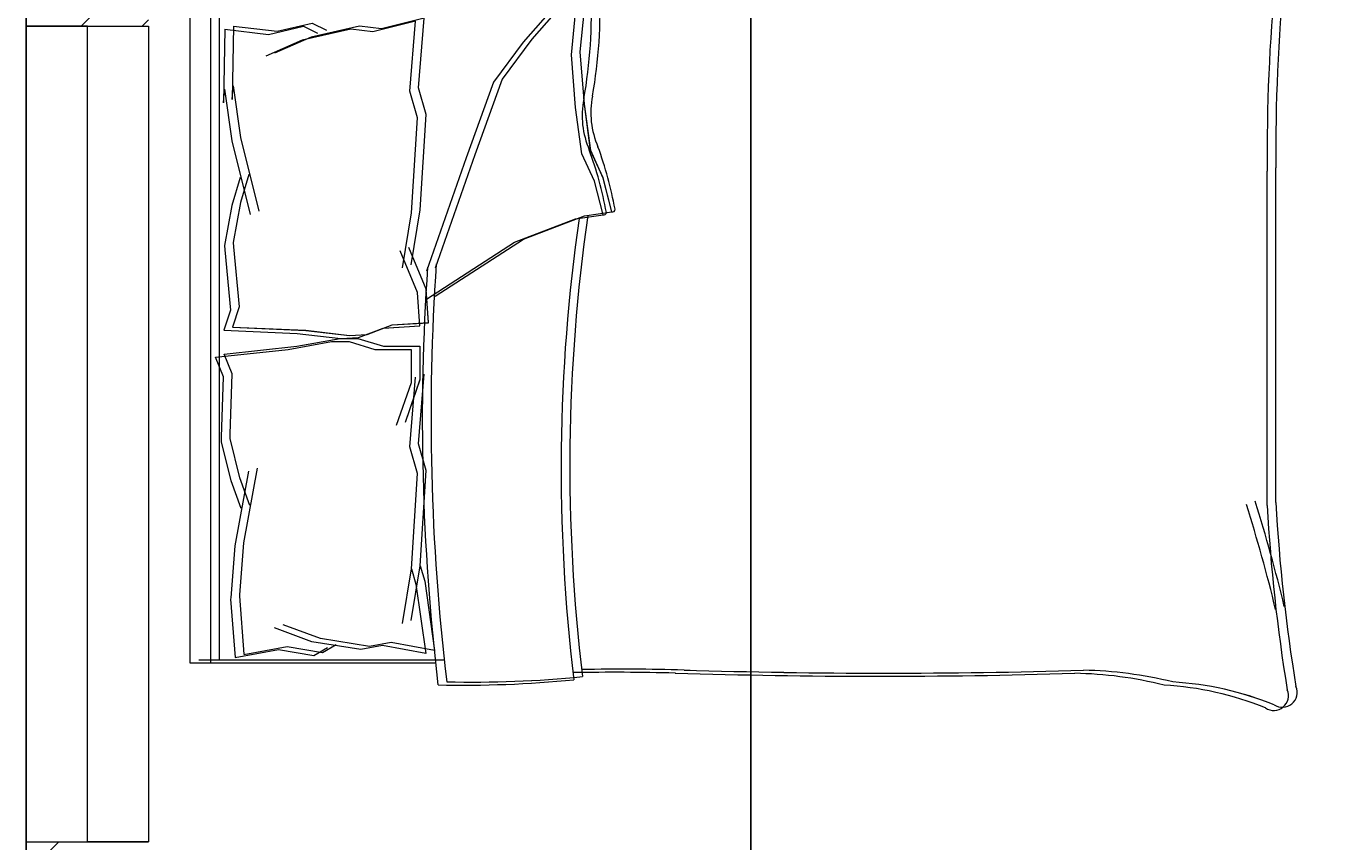
# Model space of a CAD drawing. Units: inches. Extents: x 1601 to 2297, y 1496 to 2631.
# Tile 7 of 57: x 1686 to 1783, y 1913 to 1973. Entities that reach past the tile are written whole.
import ezdxf

# ---------------------------------------------------------------- set-up
doc = ezdxf.new("R2010")
doc.units = ezdxf.units.IN
for name, color, linetype, lineweight in [('A-ANNO-DIMS', 2, 'Continuous', 18), ('A-FURN', 8, 'Continuous', 18), ('A-GLAZ', 161, 'Continuous', 20), ('A-WALL-PATT', 215, 'Continuous', 13)]:
    doc.layers.add(name, color=color, linetype=linetype, lineweight=lineweight)
doc.styles.get("Standard").update_dxf_attribs({"font": 'arial.ttf'})
doc.dimstyles.get("Standard").update_dxf_attribs({"dimtxt": 0.18, "dimasz": 0.18, "dimexe": 0.18, "dimexo": 0.0625, "dimgap": 0.09, "dimtad": 0, "dimtih": 1, "dimtoh": 1, "dimdec": 4, "dimzin": 0, "dimdsep": 46, "dimtxsty": 'Standard', "dimcen": 0.09, "dimadec": 0, "dimazin": 0, "dimtfac": 1, "dimtdec": 4, "dimtofl": 0, "dimtmove": 0, "dimatfit": 3, "dimfxl": 1, "dimtolj": 1, "dimtzin": 0, "dimarcsym": 0})

# ---------------------------------------------------------------- blocks, each defined once
blk = doc.blocks.new('BED-DOUBLE')
for p, q in [((28.385, 53.096), (25.135, 49.39)), ((28.385, 53.096), (25.135, 49.39)), ((28.385, 53.096), (25.135, 49.39)), ((28.385, 53.096), (25.135, 49.39)), ((30.13, 53.175), (28.385, 53.096, 3.871)), ((30.13, 53.175), (28.385, 53.096, 3.871)), ((30.13, 53.175), (28.385, 53.096, 3.871)), ((30.13, 53.175), (28.385, 53.096, 3.871)), ((29.004, 51.559), (28.385, 53.096)), ((29.004, 51.558), (28.385, 53.096)), ((29.004, 51.559), (28.385, 53.096)), ((29.004, 51.558), (28.385, 53.096)), ((27.746, 52.867), (24.495, 49.162)), ((27.746, 52.867), (24.495, 49.162)), ((27.746, 52.867), (24.495, 49.162)), ((27.746, 52.867), (24.495, 49.162)), ((29.49, 52.947), (27.746, 52.867, 3.871)), ((29.49, 52.947), (27.746, 52.867, 3.871)), ((29.49, 52.947), (27.746, 52.867, 3.871)), ((29.49, 52.947), (27.746, 52.867, 3.871)), ((28.365, 51.33), (27.746, 52.867)), ((28.365, 51.33), (27.746, 52.867)), ((28.365, 51.33), (27.746, 52.867)), ((28.365, 51.33), (27.746, 52.867)), ((0, 51.494), (0.639, 51.493)), ((0, 3.475), (0, 51.494)), ((0, 51.494), (0.639, 51.493)), ((0, 3.475), (0, 51.494)), ((0, 51.265), (26.61, 51.265)), ((0, 51.265), (26.61, 51.265)), ((0, 51.265), (26.61, 51.265)), ((0, 51.265), (26.61, 51.265)), ((0.639, 51.494), (27.249, 51.494)), ((0.639, 51.494), (27.249, 51.494)), ((0.639, 51.493), (27.249, 51.493)), ((0.639, 51.493), (27.249, 51.493)), ((1.533, 3.475), (1.533, 51.265)), ((1.533, 3.475), (1.533, 51.265)), ((1.533, 3.475), (1.533, 51.265)), ((1.533, 3.475), (1.533, 51.265)), ((2.173, 3.703), (2.173, 51.494)), ((2.173, 3.703), (2.173, 51.494)), ((2.173, 3.703), (2.173, 51.493)), ((2.173, 3.703), (2.173, 51.493)), ((28.055, 48.233), (28.365, 51.33)), ((28.055, 48.233), (28.365, 51.33)), ((28.055, 48.233), (28.365, 51.33)), ((28.055, 48.233), (28.365, 51.33)), ((28.695, 48.461), (29.004, 51.559)), ((28.695, 48.461), (29.004, 51.559)), ((28.695, 48.461), (29.004, 51.558)), ((28.695, 48.461), (29.004, 51.558)), ((3.196, 50.34), (3.099, 44.938)), ((3.196, 50.34), (3.099, 44.938)), ((3.196, 50.34), (3.099, 44.938)), ((3.196, 50.34), (3.099, 44.938)), ((3.196, 50.34), (6.407, 49.961)), ((3.196, 50.34), (6.407, 49.961)), ((3.196, 50.34), (6.407, 49.961)), ((3.196, 50.34), (6.407, 49.961)), ((5.768, 49.733), (8.338, 50.328)), ((5.768, 49.733), (8.338, 50.328)), ((5.768, 49.733), (8.338, 50.328)), ((5.768, 49.733), (8.338, 50.328)), ((6.407, 49.961), (8.977, 50.557)), ((6.407, 49.961), (8.977, 50.557)), ((6.407, 49.961), (8.977, 50.556)), ((6.407, 49.961), (8.977, 50.556)), ((8.338, 50.328), (9.384, 49.814)), ((8.338, 50.328), (9.384, 49.814)), ((8.338, 50.328), (9.384, 49.814)), ((8.338, 50.328), (9.384, 49.814)), ((12.468, 50.34), (8.896, 49.538)), ((12.468, 50.34), (8.896, 49.537)), ((12.468, 50.34), (8.896, 49.538)), ((12.468, 50.34), (8.896, 49.537)), ((8.977, 50.557), (10.024, 50.043)), ((8.977, 50.557), (10.024, 50.043)), ((8.977, 50.556), (10.024, 50.042)), ((8.977, 50.556), (10.024, 50.042)), ((14.073, 50.151), (12.468, 50.34)), ((14.073, 50.151), (12.468, 50.34)), ((14.073, 50.151), (12.468, 50.34)), ((14.073, 50.151), (12.468, 50.34)), ((16.573, 50.698), (13.434, 49.923)), ((16.573, 50.698), (13.434, 49.922)), ((16.573, 50.698), (13.434, 49.923)), ((16.573, 50.698), (13.434, 49.922)), ((17.212, 50.926), (14.073, 50.151)), ((17.212, 50.926), (14.073, 50.151)), ((17.212, 50.926), (14.073, 50.151)), ((17.212, 50.926), (14.073, 50.151)), ((16.169, 45.566), (16.573, 50.698)), ((16.169, 45.566), (16.573, 50.698)), ((16.169, 45.566), (16.573, 50.698)), ((16.169, 45.566), (16.573, 50.698)), ((16.808, 45.795), (17.212, 50.926)), ((16.808, 45.794), (17.212, 50.926)), ((16.808, 45.795), (17.212, 50.926)), ((16.808, 45.794), (17.212, 50.926)), ((2.557, 50.112), (2.46, 44.709)), ((2.557, 50.112), (2.46, 44.709)), ((2.557, 50.111), (2.46, 44.709)), ((2.557, 50.111), (2.46, 44.709)), ((2.557, 50.112), (5.768, 49.733)), ((2.557, 50.112), (5.768, 49.733)), ((2.557, 50.111), (5.768, 49.733)), ((2.557, 50.111), (5.768, 49.733)), ((8.257, 49.309), (5.578, 48.128)), ((8.257, 49.309), (5.578, 48.128)), ((8.257, 49.309), (5.578, 48.128)), ((8.257, 49.309), (5.578, 48.128)), ((8.896, 49.538), (6.218, 48.356)), ((8.896, 49.538), (6.218, 48.356)), ((8.896, 49.537), (6.218, 48.356)), ((8.896, 49.537), (6.218, 48.356)), ((11.829, 50.112), (8.257, 49.309)), ((11.829, 50.112), (8.257, 49.309)), ((11.829, 50.112), (8.257, 49.309)), ((11.829, 50.112), (8.257, 49.309)), ((13.434, 49.923), (11.829, 50.112)), ((13.434, 49.922), (11.829, 50.112)), ((13.434, 49.923), (11.829, 50.112)), ((13.434, 49.922), (11.829, 50.112)), ((25.135, 49.39), (22.968, 46.448)), ((25.135, 49.39), (22.968, 46.448)), ((25.135, 49.39), (22.968, 46.448)), ((25.135, 49.39), (22.968, 46.448)), ((24.495, 49.162), (22.329, 46.219)), ((24.495, 49.162), (22.329, 46.219)), ((24.495, 49.162), (22.329, 46.219)), ((24.495, 49.162), (22.329, 46.219)), ((29.004, 44.589), (28.695, 48.461)), ((29.004, 44.589), (28.695, 48.461)), ((29.004, 44.589), (28.695, 48.461)), ((29.004, 44.589), (28.695, 48.461)), ((28.365, 44.361), (28.055, 48.233)), ((28.365, 44.361), (28.055, 48.233)), ((28.365, 44.361), (28.055, 48.233)), ((28.365, 44.361), (28.055, 48.233)), ((22.968, 46.448), (20.956, 40.872)), ((22.968, 46.448), (20.956, 40.872)), ((22.968, 46.448), (20.956, 40.872)), ((22.968, 46.448), (20.956, 40.872)), ((2.46, 44.709), (2.542, 45.712)), ((2.46, 44.709), (2.542, 45.712)), ((2.46, 44.709), (2.542, 45.712)), ((2.46, 44.709), (2.542, 45.712)), ((2.542, 45.712), (3.069, 41.914)), ((2.542, 45.712), (3.069, 41.914)), ((2.542, 45.712), (3.069, 41.914)), ((2.542, 45.712), (3.069, 41.914)), ((3.099, 44.938), (3.181, 45.941)), ((3.099, 44.938), (3.181, 45.941)), ((3.099, 44.938), (3.181, 45.94)), ((3.099, 44.938), (3.181, 45.94)), ((3.181, 45.941), (3.709, 42.143)), ((3.181, 45.941), (3.709, 42.143)), ((3.181, 45.94), (3.709, 42.142)), ((3.181, 45.94), (3.709, 42.142)), ((16.726, 43.606), (16.169, 45.566)), ((16.726, 43.606), (16.169, 45.566)), ((16.726, 43.606), (16.169, 45.566)), ((16.726, 43.606), (16.169, 45.566)), ((17.365, 43.834), (16.808, 45.795)), ((17.365, 43.834), (16.808, 45.795)), ((17.365, 43.834), (16.808, 45.794)), ((17.365, 43.834), (16.808, 45.794)), ((22.329, 46.219), (20.316, 40.644)), ((22.329, 46.219), (20.316, 40.644)), ((22.329, 46.219), (20.317, 40.644)), ((22.329, 46.219), (20.317, 40.644)), ((29.468, 41.182), (29.004, 44.589)), ((29.469, 41.182), (29.004, 44.589)), ((29.468, 41.182), (29.004, 44.589)), ((29.469, 41.182), (29.004, 44.589)), ((16.295, 36.596), (16.726, 43.606)), ((16.295, 36.596), (16.726, 43.606)), ((16.295, 36.596), (16.726, 43.606)), ((16.295, 36.596), (16.726, 43.606)), ((16.934, 36.824), (17.365, 43.834)), ((16.934, 36.824), (17.365, 43.834)), ((16.934, 36.824), (17.365, 43.834)), ((16.934, 36.824), (17.365, 43.834)), ((28.829, 40.954), (28.365, 44.361)), ((28.829, 40.953), (28.365, 44.361)), ((28.829, 40.954), (28.365, 44.361)), ((28.829, 40.953), (28.365, 44.361)), ((3.069, 41.914), (4.422, 36.495)), ((3.069, 41.914), (4.422, 36.495)), ((3.069, 41.914), (4.422, 36.495)), ((3.069, 41.914), (4.422, 36.495)), ((3.709, 42.143), (5.061, 36.723)), ((3.709, 42.143), (5.061, 36.723)), ((3.709, 42.142), (5.061, 36.723)), ((3.709, 42.142), (5.061, 36.723)), ((20.316, 40.644), (17.383, 32.306)), ((20.317, 40.644), (17.383, 32.306)), ((20.316, 40.644), (17.383, 32.306)), ((20.317, 40.644), (17.383, 32.306)), ((20.956, 40.872), (18.022, 32.534)), ((20.956, 40.872), (18.022, 32.534)), ((20.956, 40.872), (18.022, 32.534)), ((20.956, 40.872), (18.022, 32.534)), ((29.758, 38.94), (28.829, 40.954)), ((29.758, 38.94), (28.829, 40.954)), ((29.758, 38.94), (28.829, 40.953)), ((29.758, 38.94), (28.829, 40.953)), ((30.397, 39.169), (29.468, 41.182)), ((30.397, 39.169), (29.468, 41.182)), ((30.397, 39.168), (29.469, 41.182)), ((30.397, 39.168), (29.469, 41.182)), ((79.245, 15.063), (79.245, 39.677)), ((79.245, 15.063), (79.245, 39.677)), ((79.245, 15.063), (79.245, 39.677)), ((79.245, 15.063), (79.245, 39.677)), ((79.884, 15.292), (79.884, 39.905)), ((79.884, 15.291), (79.884, 39.905)), ((79.884, 15.292), (79.884, 39.905)), ((79.884, 15.291), (79.884, 39.905)), ((3.673, 39.2), (3.078, 37.135)), ((3.673, 39.2), (3.078, 37.135)), ((3.673, 39.2), (3.078, 37.135)), ((3.673, 39.2), (3.078, 37.135)), ((4.313, 39.428), (3.717, 37.363)), ((4.313, 39.428), (3.717, 37.363)), ((4.313, 39.428), (3.718, 37.363)), ((4.313, 39.428), (3.718, 37.363)), ((30.377, 36.462), (29.758, 38.94)), ((30.377, 36.462), (29.758, 38.94)), ((30.377, 36.462), (29.758, 38.94)), ((30.377, 36.462), (29.758, 38.94)), ((31.016, 36.691), (30.397, 39.169)), ((31.016, 36.691), (30.397, 39.169)), ((31.016, 36.691), (30.397, 39.168)), ((31.016, 36.691), (30.397, 39.168)), ((3.078, 37.135), (2.537, 34.204)), ((3.078, 37.135), (2.537, 34.204)), ((3.078, 37.135), (2.537, 34.204)), ((3.078, 37.135), (2.537, 34.204)), ((3.717, 37.363), (3.176, 34.433)), ((3.718, 37.363), (3.176, 34.433)), ((3.717, 37.363), (3.176, 34.433)), ((3.718, 37.363), (3.176, 34.433)), ((16.268, 32.792), (16.934, 36.824)), ((16.268, 32.792), (16.934, 36.824)), ((16.268, 32.792), (16.934, 36.824)), ((16.268, 32.792), (16.934, 36.824)), ((29.004, 36.381), (31.016, 36.691)), ((29.004, 36.381), (31.016, 36.691)), ((29.004, 36.381), (31.016, 36.691)), ((29.004, 36.381), (31.016, 36.691)), ((15.628, 32.564), (16.295, 36.596)), ((15.628, 32.564), (16.295, 36.596)), ((15.628, 32.564), (16.295, 36.596)), ((15.628, 32.564), (16.295, 36.596)), ((23.876, 34.449), (28.365, 36.153)), ((23.876, 34.449), (28.365, 36.153)), ((23.876, 34.449), (28.365, 36.152)), ((23.876, 34.449), (28.365, 36.152)), ((24.516, 34.677), (29.004, 36.381)), ((24.516, 34.677), (29.004, 36.381)), ((24.516, 34.677), (29.004, 36.381)), ((24.516, 34.677), (29.004, 36.381)), ((28.365, 36.153), (30.377, 36.462)), ((28.365, 36.152), (30.377, 36.462)), ((28.365, 36.153), (30.377, 36.462)), ((28.365, 36.152), (30.377, 36.462)), ((2.537, 34.204), (2.557, 33.883)), ((2.537, 34.204), (2.557, 33.883)), ((2.537, 34.204), (2.557, 33.883)), ((2.537, 34.204), (2.557, 33.883)), ((2.557, 33.883), (2.979, 29.456)), ((2.557, 33.883), (2.979, 29.455)), ((2.557, 33.883), (2.979, 29.456)), ((2.557, 33.883), (2.979, 29.455)), ((3.176, 34.433), (3.196, 34.112)), ((3.176, 34.433), (3.196, 34.112)), ((3.176, 34.433), (3.196, 34.112)), ((3.176, 34.433), (3.196, 34.112)), ((3.196, 34.112), (3.618, 29.684)), ((3.196, 34.112), (3.618, 29.684)), ((3.196, 34.112), (3.618, 29.684)), ((3.196, 34.112), (3.618, 29.684)), ((16.739, 30.75), (15.454, 33.821)), ((16.739, 30.75), (15.454, 33.821)), ((16.739, 30.75), (15.454, 33.82)), ((16.739, 30.75), (15.454, 33.82)), ((17.379, 30.978), (16.094, 34.049)), ((17.379, 30.978), (16.094, 34.049)), ((17.379, 30.978), (16.094, 34.049)), ((17.379, 30.978), (16.094, 34.049)), ((17.383, 30.259), (23.876, 34.449)), ((17.383, 30.259), (23.876, 34.449)), ((17.383, 30.259), (23.876, 34.449)), ((17.383, 30.259), (23.876, 34.449)), ((18.022, 30.487), (24.516, 34.677)), ((18.022, 30.487), (24.516, 34.677)), ((18.022, 30.487), (24.516, 34.677)), ((18.022, 30.487), (24.516, 34.677)), ((17.532, 28.526), (17.379, 30.978)), ((17.532, 28.525), (17.379, 30.978)), ((17.532, 28.526), (17.379, 30.978)), ((17.532, 28.525), (17.379, 30.978)), ((16.893, 28.297), (16.739, 30.75)), ((16.893, 28.297), (16.739, 30.75)), ((16.893, 28.297), (16.739, 30.75)), ((16.893, 28.297), (16.739, 30.75)), ((2.979, 29.456), (2.492, 27.977)), ((2.979, 29.456), (2.492, 27.977)), ((2.979, 29.455), (2.492, 27.976)), ((2.979, 29.455), (2.492, 27.976)), ((3.618, 29.684), (3.131, 28.205)), ((3.618, 29.684), (3.131, 28.205)), ((3.618, 29.684), (3.131, 28.205)), ((3.618, 29.684), (3.131, 28.205)), ((3.131, 28.205), (8.506, 27.962)), ((3.131, 28.205), (8.506, 27.961)), ((3.131, 28.205), (8.506, 27.962)), ((3.131, 28.205), (8.506, 27.961)), ((12.377, 27.436), (14.216, 28.13)), ((12.377, 27.436), (14.217, 28.13)), ((12.377, 27.436), (14.216, 28.13)), ((12.377, 27.436), (14.217, 28.13)), ((13.016, 27.664), (14.856, 28.359)), ((13.016, 27.664), (14.856, 28.359)), ((13.016, 27.664), (14.856, 28.358)), ((13.016, 27.664), (14.856, 28.358)), ((14.216, 28.13), (16.893, 28.297)), ((14.216, 28.13), (16.893, 28.297)), ((14.217, 28.13), (16.893, 28.297)), ((14.217, 28.13), (16.893, 28.297)), ((14.856, 28.359), (17.532, 28.526)), ((14.856, 28.359), (17.532, 28.526)), ((14.856, 28.358), (17.532, 28.525)), ((14.856, 28.358), (17.532, 28.525)), ((2.492, 27.977), (7.867, 27.733)), ((2.492, 27.977), (7.867, 27.733)), ((2.492, 27.976), (7.867, 27.733)), ((2.492, 27.976), (7.867, 27.733)), ((7.22, 26.561), (10.401, 27.139)), ((7.22, 26.56), (10.401, 27.139)), ((7.22, 26.561), (10.401, 27.139)), ((7.22, 26.56), (10.401, 27.139)), ((7.859, 26.789), (11.04, 27.367)), ((7.859, 26.789), (11.04, 27.367)), ((7.859, 26.789), (11.04, 27.367)), ((7.859, 26.789), (11.04, 27.367)), ((7.867, 27.733), (11.078, 27.355)), ((7.867, 27.733), (11.078, 27.354)), ((7.867, 27.733), (11.078, 27.355)), ((7.867, 27.733), (11.078, 27.354)), ((8.506, 27.962), (11.717, 27.583)), ((8.506, 27.962), (11.717, 27.583)), ((8.506, 27.961), (11.717, 27.583)), ((8.506, 27.961), (11.717, 27.583)), ((10.401, 27.139), (11.702, 27.139)), ((10.401, 27.139), (11.702, 27.139)), ((10.401, 27.139), (11.702, 27.139)), ((10.401, 27.139), (11.702, 27.139)), ((11.04, 27.367), (12.341, 27.367)), ((11.04, 27.367), (12.341, 27.367)), ((11.04, 27.367), (12.341, 27.367)), ((11.04, 27.367), (12.341, 27.367)), ((11.078, 27.355), (12.377, 27.436)), ((11.078, 27.354), (12.377, 27.436)), ((11.078, 27.355), (12.377, 27.436)), ((11.078, 27.354), (12.377, 27.436)), ((11.702, 27.139), (13.582, 26.561)), ((11.702, 27.139), (13.582, 26.56)), ((11.702, 27.139), (13.582, 26.561)), ((11.702, 27.139), (13.582, 26.56)), ((11.717, 27.583), (13.016, 27.664)), ((11.717, 27.583), (13.016, 27.664)), ((11.717, 27.583), (13.016, 27.664)), ((11.717, 27.583), (13.016, 27.664)), ((12.341, 27.367), (14.221, 26.789)), ((12.341, 27.367), (14.221, 26.789)), ((12.341, 27.367), (14.221, 26.789)), ((12.341, 27.367), (14.221, 26.789)), ((1.87, 25.982), (7.22, 26.561)), ((1.87, 25.982), (7.22, 26.561)), ((1.87, 25.982), (7.22, 26.56)), ((1.87, 25.982), (7.22, 26.56)), ((2.509, 26.211), (7.859, 26.789)), ((2.509, 26.21), (7.859, 26.789)), ((2.509, 26.211), (7.859, 26.789)), ((2.509, 26.21), (7.859, 26.789)), ((3.088, 24.765), (2.509, 26.211)), ((3.088, 24.765), (2.509, 26.211)), ((3.088, 24.765), (2.509, 26.21)), ((3.088, 24.765), (2.509, 26.21)), ((13.582, 26.561), (16.263, 26.561)), ((13.582, 26.561), (16.263, 26.561)), ((13.582, 26.56), (16.263, 26.56)), ((13.582, 26.56), (16.263, 26.56)), ((14.221, 26.789), (16.902, 26.789)), ((14.221, 26.789), (16.902, 26.789)), ((14.221, 26.789), (16.902, 26.789)), ((14.221, 26.789), (16.902, 26.789)), ((16.263, 26.561), (16.263, 24.103)), ((16.263, 26.561), (16.263, 24.103)), ((16.263, 26.56), (16.263, 24.103)), ((16.263, 26.56), (16.263, 24.103)), ((16.902, 26.789), (16.902, 24.332)), ((16.902, 26.789), (16.902, 24.331)), ((16.902, 26.789), (16.902, 24.332)), ((16.902, 26.789), (16.902, 24.331)), ((2.448, 24.537), (1.87, 25.982)), ((2.448, 24.537), (1.87, 25.982)), ((2.448, 24.537), (1.87, 25.982)), ((2.448, 24.537), (1.87, 25.982)), ((2.304, 20.091), (2.448, 24.537)), ((2.304, 20.091), (2.448, 24.537)), ((2.304, 20.091), (2.448, 24.537)), ((2.304, 20.091), (2.448, 24.537)), ((2.943, 20.32), (3.088, 24.765)), ((2.943, 20.319), (3.088, 24.765)), ((2.943, 20.32), (3.088, 24.765)), ((2.943, 20.319), (3.088, 24.765)), ((16.902, 24.332), (15.811, 21.187)), ((16.902, 24.332), (15.811, 21.187)), ((16.902, 24.331), (15.811, 21.187)), ((16.902, 24.331), (15.811, 21.187)), ((16.169, 19.384), (16.573, 24.516)), ((16.169, 19.384), (16.573, 24.516)), ((16.169, 19.383), (16.573, 24.515)), ((16.169, 19.383), (16.573, 24.515)), ((16.808, 19.612), (17.212, 24.744)), ((16.808, 19.612), (17.212, 24.744)), ((16.808, 19.612), (17.212, 24.744)), ((16.808, 19.612), (17.212, 24.744)), ((16.263, 24.103), (15.172, 20.959)), ((16.263, 24.103), (15.172, 20.958)), ((16.263, 24.103), (15.172, 20.959)), ((16.263, 24.103), (15.172, 20.958)), ((2.943, 19.998), (2.943, 20.32)), ((2.943, 19.998), (2.943, 20.32)), ((2.943, 19.998), (2.943, 20.319)), ((2.943, 19.998), (2.943, 20.319)), ((2.304, 19.77), (2.304, 20.091)), ((2.304, 19.769), (2.304, 20.091)), ((2.304, 19.77), (2.304, 20.091)), ((2.304, 19.769), (2.304, 20.091)), ((3.027, 16.878), (2.304, 19.77)), ((3.027, 16.878), (2.304, 19.77)), ((3.027, 16.878), (2.304, 19.769)), ((3.027, 16.878), (2.304, 19.769)), ((3.666, 17.107), (2.943, 19.998)), ((3.666, 17.107), (2.943, 19.998)), ((3.666, 17.107), (2.943, 19.998)), ((3.666, 17.107), (2.943, 19.998)), ((16.726, 17.423), (16.169, 19.384)), ((16.726, 17.423), (16.169, 19.384)), ((16.726, 17.423), (16.169, 19.383)), ((16.726, 17.423), (16.169, 19.383)), ((17.365, 17.652), (16.808, 19.612)), ((17.365, 17.651), (16.808, 19.612)), ((17.365, 17.652), (16.808, 19.612)), ((17.365, 17.651), (16.808, 19.612)), ((3.316, 12.108), (4.328, 17.601)), ((3.316, 12.108), (4.328, 17.601)), ((3.316, 12.108), (4.328, 17.601)), ((3.316, 12.108), (4.328, 17.601)), ((3.955, 12.336), (4.967, 17.83)), ((3.955, 12.336), (4.967, 17.83)), ((3.955, 12.336), (4.967, 17.829)), ((3.955, 12.336), (4.967, 17.829)), ((16.295, 10.413), (16.726, 17.423)), ((16.295, 10.413), (16.726, 17.423)), ((16.295, 10.413), (16.726, 17.423)), ((16.295, 10.413), (16.726, 17.423)), ((16.934, 10.642), (17.365, 17.652)), ((16.934, 10.642), (17.365, 17.652)), ((16.934, 10.642), (17.365, 17.651)), ((16.934, 10.642), (17.365, 17.651)), ((3.75, 14.855), (3.027, 16.878)), ((3.75, 14.854), (3.027, 16.878)), ((3.75, 14.855), (3.027, 16.878)), ((3.75, 14.854), (3.027, 16.878)), ((4.389, 15.083), (3.666, 17.107)), ((4.389, 15.083), (3.666, 17.107)), ((4.389, 15.083), (3.666, 17.107)), ((4.389, 15.083), (3.666, 17.107)), ((3.027, 8.285), (3.316, 12.108)), ((3.027, 8.284), (3.316, 12.108)), ((3.027, 8.285), (3.316, 12.108)), ((3.027, 8.284), (3.316, 12.108)), ((3.666, 8.513), (3.955, 12.336)), ((3.666, 8.513), (3.955, 12.336)), ((3.666, 8.513), (3.955, 12.336)), ((3.666, 8.513), (3.955, 12.336)), ((16.268, 6.61), (16.934, 10.642)), ((16.268, 6.61), (16.934, 10.642)), ((16.268, 6.61), (16.934, 10.642)), ((16.268, 6.61), (16.934, 10.642)), ((16.934, 10.642), (17.257, 9.509)), ((16.934, 10.642), (17.257, 9.508)), ((16.934, 10.642), (17.257, 9.509)), ((16.934, 10.642), (17.257, 9.508)), ((15.628, 6.382), (16.295, 10.413)), ((15.628, 6.381), (16.295, 10.413)), ((15.628, 6.382), (16.295, 10.413)), ((15.628, 6.381), (16.295, 10.413)), ((16.295, 10.413), (16.618, 9.28)), ((16.295, 10.413), (16.618, 9.28)), ((16.295, 10.413), (16.618, 9.28)), ((16.295, 10.413), (16.618, 9.28)), ((16.618, 9.28), (17.341, 4.184)), ((16.618, 9.28), (17.341, 4.183)), ((16.618, 9.28), (17.341, 4.184)), ((16.618, 9.28), (17.341, 4.183)), ((17.257, 9.509), (17.98, 4.412)), ((17.257, 9.509), (17.98, 4.412)), ((17.257, 9.508), (17.98, 4.412)), ((17.257, 9.508), (17.98, 4.412)), ((3.009, 8.179), (3.027, 8.285)), ((3.009, 8.179), (3.027, 8.285)), ((3.009, 8.179), (3.027, 8.284)), ((3.009, 8.179), (3.027, 8.284)), ((3.338, 3.898), (3.009, 8.179)), ((3.338, 3.898), (3.009, 8.179)), ((3.338, 3.898), (3.009, 8.179)), ((3.338, 3.898), (3.009, 8.179)), ((3.648, 8.408), (3.666, 8.513)), ((3.648, 8.407), (3.666, 8.513)), ((3.648, 8.408), (3.666, 8.513)), ((3.648, 8.407), (3.666, 8.513)), ((3.977, 4.127), (3.648, 8.408)), ((3.977, 4.127), (3.648, 8.408)), ((3.977, 4.127), (3.648, 8.407)), ((3.977, 4.127), (3.648, 8.407)), ((8.955, 5.051), (6.208, 6.063)), ((8.955, 5.051), (6.208, 6.063)), ((8.955, 5.051), (6.208, 6.063)), ((8.955, 5.051), (6.208, 6.063)), ((9.594, 5.279), (6.847, 6.291)), ((9.594, 5.279), (6.847, 6.291)), ((9.594, 5.279), (6.847, 6.291)), ((9.594, 5.279), (6.847, 6.291)), ((12.57, 4.473), (8.955, 5.051)), ((12.57, 4.472), (8.955, 5.051)), ((12.57, 4.473), (8.955, 5.051)), ((12.57, 4.472), (8.955, 5.051)), ((13.209, 4.701), (9.594, 5.279)), ((13.209, 4.701), (9.594, 5.279)), ((13.209, 4.701), (9.594, 5.279)), ((13.209, 4.701), (9.594, 5.279)), ((9.739, 4.267), (10.751, 4.846)), ((9.739, 4.267), (10.751, 4.846)), ((9.739, 4.267), (10.751, 4.845)), ((9.739, 4.267), (10.751, 4.845)), ((14.799, 4.99), (13.209, 4.701)), ((14.799, 4.99), (13.209, 4.701)), ((14.799, 4.99), (13.209, 4.701)), ((14.799, 4.99), (13.209, 4.701)), ((17.98, 4.412), (14.799, 4.99)), ((17.98, 4.412), (14.799, 4.99)), ((17.98, 4.412), (14.799, 4.99)), ((17.98, 4.412), (14.799, 4.99)), ((3.316, 3.894), (6.497, 4.473)), ((3.316, 3.894), (6.497, 4.473)), ((3.316, 3.894), (6.497, 4.472)), ((3.316, 3.894), (6.497, 4.472)), ((3.955, 4.123), (7.136, 4.701)), ((3.955, 4.123), (7.136, 4.701)), ((3.955, 4.123), (7.136, 4.701)), ((3.955, 4.123), (7.136, 4.701)), ((6.497, 4.473), (9.099, 4.039)), ((6.497, 4.473), (9.099, 4.039)), ((6.497, 4.472), (9.099, 4.039)), ((6.497, 4.472), (9.099, 4.039)), ((7.136, 4.701), (9.739, 4.267)), ((7.136, 4.701), (9.739, 4.267)), ((7.136, 4.701), (9.739, 4.267)), ((7.136, 4.701), (9.739, 4.267)), ((9.099, 4.039), (10.112, 4.617)), ((9.099, 4.039), (10.112, 4.617)), ((9.099, 4.039), (10.112, 4.617)), ((9.099, 4.039), (10.112, 4.617)), ((14.16, 4.762), (12.57, 4.473)), ((14.16, 4.762), (12.57, 4.472)), ((14.16, 4.762), (12.57, 4.473)), ((14.16, 4.762), (12.57, 4.472)), ((17.341, 4.184), (14.16, 4.762)), ((17.341, 4.183), (14.16, 4.762)), ((17.341, 4.184), (14.16, 4.762)), ((17.341, 4.183), (14.16, 4.762)), ((18.11, 3.475), (0, 3.475)), ((18.11, 3.475), (0, 3.475)), ((18.11, 3.475), (0, 3.475)), ((18.11, 3.475), (0, 3.475)), ((18.75, 3.703), (0.639, 3.703)), ((18.75, 3.703), (0.639, 3.703)), ((18.75, 3.703), (0.639, 3.703)), ((18.75, 3.703), (0.639, 3.703))]:
    blk.add_line(p, q)
for centre, radius, start, end in [((68.666, 76.157), 23.065, 267.47136, 296.46809), ((68.666, 76.157), 23.065, 267.47136, 296.46809), ((68.666, 76.157), 23.065, 267.47136, 296.46809), ((68.666, 76.157), 23.065, 267.47136, 296.46809), ((69.306, 76.385), 23.065, 267.47136, 296.46809), ((69.306, 76.385), 23.065, 267.47136, 296.46809), ((69.306, 76.385), 23.065, 267.47136, 296.46809), ((69.306, 76.385), 23.065, 267.47136, 296.46809), ((78.87, 54.41), 1.102, 332.65876, 86.02002), ((78.87, 54.409), 1.102, 332.65876, 86.02002), ((78.87, 54.41), 1.102, 332.65876, 86.02002), ((78.87, 54.409), 1.102, 332.65876, 86.02002), ((79.509, 54.638), 1.102, 332.65876, 86.02002), ((79.509, 54.638), 1.102, 332.65876, 86.02002), ((79.509, 54.638), 1.102, 332.65876, 86.02002), ((79.509, 54.638), 1.102, 332.65876, 86.02002), ((212.916, 41.38), 133.04, 174.4998, 180.63509), ((212.916, 41.38), 133.04, 174.4998, 180.63509), ((212.916, 41.38), 133.04, 174.4998, 180.63509), ((212.916, 41.38), 133.04, 174.4998, 180.63509), ((-6.017, 51.555), 36.183, 349.87628, 2.56571), ((-6.017, 51.555), 36.183, 349.87628, 2.56571), ((-6.017, 51.555), 36.183, 349.87628, 2.56571), ((-6.017, 51.555), 36.183, 349.87628, 2.56571), ((36.954, 182.494), 129.499, 266.97912, 273.83645), ((36.954, 182.494), 129.499, 266.97912, 273.83645), ((36.954, 182.494), 129.499, 266.97912, 273.83645), ((36.954, 182.494), 129.499, 266.97912, 273.83645), ((67.821, -4508.744), 4561.858, 90.002168, 90.286887), ((67.821, -4508.744), 4561.858, 90.002168, 90.286887), ((67.821, -4508.744), 4561.858, 90.002168, 90.286887), ((67.821, -4508.744), 4561.858, 90.002168, 90.286887), ((68.461, -4508.515), 4561.858, 90.002168, 90.286887), ((68.461, -4508.515), 4561.858, 90.002168, 90.286887), ((68.461, -4508.516), 4561.858, 90.002168, 90.286887), ((68.461, -4508.516), 4561.858, 90.002168, 90.286887), ((212.276, 41.152), 133.04, 174.4998, 180.63509), ((212.277, 41.151), 133.04, 174.4998, 180.63509), ((212.276, 41.152), 133.04, 174.4998, 180.63509), ((212.277, 41.151), 133.04, 174.4998, 180.63509), ((-6.656, 51.327), 36.183, 349.87628, 2.56571), ((-6.656, 51.327), 36.183, 349.87628, 2.56571), ((-6.656, 51.327), 36.183, 349.87628, 2.56571), ((-6.656, 51.327), 36.183, 349.87628, 2.56571), ((36.315, 182.266), 129.499, 266.97912, 273.83645), ((36.315, 182.265), 129.499, 266.97912, 273.83645), ((36.315, 182.266), 129.499, 266.97912, 273.83645), ((36.315, 182.265), 129.499, 266.97912, 273.83645), ((35.066, 43.743), 6.224, 168.6608, 203.73842), ((35.066, 43.743), 6.224, 168.6608, 203.73842), ((35.066, 43.743), 6.224, 168.6608, 203.73842), ((35.066, 43.743), 6.224, 168.6608, 203.73842), ((35.705, 43.972), 6.224, 168.6608, 203.73842), ((35.705, 43.971), 6.224, 168.6608, 203.73842), ((35.705, 43.972), 6.224, 168.6608, 203.73842), ((35.705, 43.971), 6.224, 168.6608, 203.73842), ((1.482, 31.154), 29.654, 10.66171, 19.88058), ((1.482, 31.154), 29.654, 10.66171, 19.88058), ((1.482, 31.153), 29.654, 10.66171, 19.88058), ((1.482, 31.153), 29.654, 10.66171, 19.88058), ((2.121, 31.382), 29.654, 10.66171, 19.88058), ((2.121, 31.382), 29.654, 10.66171, 19.88058), ((2.121, 31.382), 29.654, 10.66171, 19.88058), ((2.121, 31.382), 29.654, 10.66171, 19.88058), ((31.079, 36.864), 0.185, 250.24637, 1.13765), ((31.079, 36.864), 0.185, 250.24637, 1.13765), ((31.079, 36.864), 0.185, 250.24637, 1.13765), ((31.079, 36.864), 0.185, 250.24637, 1.13765), ((156.316, 17.756), 129.02, 171.78449, 186.90062), ((156.316, 17.755), 129.02, 171.78449, 186.90062), ((156.316, 17.756), 129.02, 171.78449, 186.90062), ((156.316, 17.755), 129.02, 171.78449, 186.90062), ((156.955, 17.984), 129.02, 171.78449, 186.90062), ((156.955, 17.984), 129.02, 171.78449, 186.90062), ((156.955, 17.984), 129.02, 171.78449, 186.90062), ((156.955, 17.984), 129.02, 171.78449, 186.90062), ((30.439, 36.636), 0.185, 250.24637, 1.13765), ((30.439, 36.636), 0.185, 250.24637, 1.13765), ((30.439, 36.636), 0.185, 250.24637, 1.13765), ((30.439, 36.636), 0.185, 250.24637, 1.13765), ((182.692, 21.587), 164.969, 176.08655, 186.78213), ((182.692, 21.587), 164.969, 176.08655, 186.78213), ((182.692, 21.587), 164.969, 176.08655, 186.78213), ((182.692, 21.587), 164.969, 176.08655, 186.78213), ((182.052, 21.359), 164.969, 176.08655, 186.78213), ((182.052, 21.359), 164.969, 176.08655, 186.78213), ((182.052, 21.358), 164.969, 176.08655, 186.78213), ((182.052, 21.358), 164.969, 176.08655, 186.78213), ((-23.712, -17.222), 106.459, 13.38322, 17.70533), ((-23.712, -17.222), 106.459, 13.38322, 17.70533), ((-23.712, -17.222), 106.459, 13.38322, 17.70533), ((-23.712, -17.222), 106.459, 13.38322, 17.70533), ((-23.073, -16.994), 106.459, 13.38322, 17.70533), ((-23.073, -16.994), 106.459, 13.38322, 17.70533), ((-23.073, -16.994), 106.459, 13.38322, 17.70533), ((-23.073, -16.994), 106.459, 13.38322, 17.70533), ((200.837, 21.427), 121.759, 182.99578, 189.40907), ((200.837, 21.426), 121.759, 182.99578, 189.40907), ((200.837, 21.427), 121.759, 182.99578, 189.40907), ((200.837, 21.426), 121.759, 182.99578, 189.40907), ((201.476, 21.655), 121.759, 182.99578, 189.40907), ((201.476, 21.655), 121.759, 182.99578, 189.40907), ((201.476, 21.655), 121.759, 182.99578, 189.40907), ((201.476, 21.655), 121.759, 182.99578, 189.40907), ((31.813, -167.079), 170.11, 88.4762, 91.00819), ((31.813, -167.08), 170.11, 88.4762, 91.00819), ((31.813, -167.079), 170.11, 88.4762, 91.00819), ((31.813, -167.08), 170.11, 88.4762, 91.00819), ((51.253, 485.051), 482.31, 268.22771, 271.71854), ((51.253, 485.05), 482.31, 268.22771, 271.71854), ((51.253, 485.051), 482.31, 268.22771, 271.71854), ((51.253, 485.05), 482.31, 268.22771, 271.71854), ((65.154, -26.671), 29.634, 76.06484, 88.91125), ((65.154, -26.672), 29.634, 76.06484, 88.91125), ((65.154, -26.671), 29.634, 76.06484, 88.91125), ((65.154, -26.672), 29.634, 76.06484, 88.91125), ((20.096, 85.162), 83.306, 268.72178, 275.60397), ((20.096, 85.161), 83.306, 268.72178, 275.60397), ((20.096, 85.162), 83.306, 268.72178, 275.60397), ((20.096, 85.161), 83.306, 268.72178, 275.60397), ((20.735, 85.39), 83.306, 268.72178, 275.60397), ((20.735, 85.39), 83.306, 268.72178, 275.60397), ((20.736, 85.39), 83.306, 268.72178, 275.60397), ((20.736, 85.39), 83.306, 268.72178, 275.60397), ((31.174, -167.308), 170.11, 88.4762, 91.00819), ((31.174, -167.308), 170.11, 88.4762, 91.00819), ((31.174, -167.308), 170.11, 88.4762, 91.00819), ((31.174, -167.308), 170.11, 88.4762, 91.00819), ((50.614, 484.822), 482.31, 268.22771, 271.71854), ((50.614, 484.822), 482.31, 268.22771, 271.71854), ((50.614, 484.822), 482.31, 268.22771, 271.71854), ((50.614, 484.822), 482.31, 268.22771, 271.71854), ((64.515, -26.9), 29.634, 76.06484, 88.91125), ((64.515, -26.9), 29.634, 76.06484, 88.91125), ((64.515, -26.9), 29.634, 76.06484, 88.91125), ((64.515, -26.9), 29.634, 76.06484, 88.91125), ((70.915, -21.431), 23.562, 67.97508, 86.652), ((70.915, -21.432), 23.562, 67.97508, 86.652), ((70.915, -21.431), 23.562, 67.97508, 86.652), ((70.915, -21.432), 23.562, 67.97508, 86.652), ((70.276, -21.66), 23.562, 67.97508, 86.652), ((70.276, -21.66), 23.562, 67.97508, 86.652), ((70.276, -21.66), 23.562, 67.97508, 86.652), ((70.276, -21.66), 23.562, 67.97508, 86.652), ((79.718, 1.087), 1.089, 236.17358, 23.47814), ((79.718, 1.087), 1.089, 236.17358, 23.47814), ((79.718, 1.087), 1.089, 236.17358, 23.47814), ((79.718, 1.087), 1.089, 236.17358, 23.47814), ((80.357, 1.316), 1.089, 236.17358, 23.47814), ((80.357, 1.316), 1.089, 236.17358, 23.47814), ((80.357, 1.315), 1.089, 236.17358, 23.47814), ((80.357, 1.315), 1.089, 236.17358, 23.47814)]:
    blk.add_arc(centre, radius, start, end)
blk = doc.blocks.new('WIN-60IN-JAMB9')
for p, q in [((4.5, 60), (0, 60)), ((0, 60), (9, 60)), ((0, 60), (0, 0)), ((4.5, 0), (4.5, 60)), ((9, 60), (9, 0)), ((0, 0), (9, 0)), ((9, 0), (4.5, 0))]:
    blk.add_line(p, q)
blk = doc.blocks.new('*D36')
at = {"layer": 'A-ANNO-DIMS', "color": 0, "lineweight": -2, "transparency": 16777216}
for p, q in [((1686.037, 1635.388), (1686.037, 2581.055)), ((1739.334, 1635.388), (1739.334, 2581.055)), ((1686.217, 2580.875), (1712.362, 2580.875)), ((1739.154, 2580.875), (1713.009, 2580.875))]:
    blk.add_line(p, q, dxfattribs=at)
at = {"layer": 'A-ANNO-DIMS', "color": 0, "transparency": 16777216}
for points in [[(1686.217, 2580.905), (1686.217, 2580.845), (1686.037, 2580.875)], [(1739.154, 2580.905), (1739.154, 2580.845), (1739.334, 2580.875)]]:
    blk.add_solid(points, dxfattribs=at)
at = {"layer": 'Defpoints', "color": 0, "transparency": 16777216}
for p in [(1739.334, 2580.875), (1686.037, 1635.325), (1739.334, 1635.325)]:
    blk.add_point(p, dxfattribs=at)
at = {"layer": 'A-ANNO-DIMS', "color": 0, "transparency": 16777216, "insert": (1712.685, 2580.875), "char_height": 0.18, "attachment_point": 5}
blk.add_mtext('\\A1;53.3', dxfattribs=at)

msp = doc.modelspace()

# ---------------------------------------------------------------- hatches: boundary and pattern name
at = {"layer": 'A-WALL-PATT'}
h = msp.add_hatch(dxfattribs=at)
h.set_pattern_fill('ANSI32', color=256)
h.paths.add_polyline_path([(2230.5373, 1861.8254), (2182.5373, 1861.8254), (2182.5373, 1885.3637), (2178.0373, 1885.3637), (2178.0373, 1861.8254), (2166.0373, 1861.8254), (2134.5373, 1861.8254), (2130.0373, 1861.8254), (2130.0373, 1841.4682), (2126.8833, 1841.4682), (2126.8833, 1836.9682), (2130.0373, 1836.9682), (2130.0373, 1822.7302), (2134.5373, 1822.7302), (2134.5373, 1857.3254), (2166.0373, 1857.3254), (2226.0373, 1857.3254), (2226.0373, 1846.1155), (2230.5373, 1846.1155)])
h.paths.add_polyline_path([(2226.0373, 1797.3254), (2134.5373, 1797.3254), (2134.5373, 1800.6636), (2132.2873, 1800.6636), (2130.0373, 1800.6636), (2130.0373, 1797.3254), (2130.0373, 1792.8254), (2167.7264, 1792.8254), (2226.0373, 1792.8254)])
h.paths.add_polyline_path([(2230.5373, 1822.1155), (2226.0373, 1822.1155), (2226.0373, 1760.8563), (2230.5373, 1760.8563)])
h.paths.add_polyline_path([(2230.5373, 1700.8563), (2226.0373, 1700.8563), (2226.0373, 1644.3254), (2140.2517, 1644.3254), (2140.2517, 1635.3254), (2230.5373, 1635.3254)])
h.paths.add_polyline_path([(2080.2517, 1639.8254), (2080.2517, 1644.3254), (2035.5373, 1644.3254), (2035.5373, 1792.8254), (2094.0373, 1792.8254), (2094.0373, 1797.3254), (2094.0373, 1836.9682), (2097.1057, 1836.9682), (2097.1057, 1839.2182), (2097.1057, 1841.4682), (2094.0373, 1841.4682), (2094.0373, 1862.2276), (2089.5373, 1862.2276), (2089.5373, 1797.3254), (2035.5373, 1797.3254), (2035.5373, 1857.3254), (2035.5373, 1885.0916), (2031.0373, 1885.0916), (2031.0373, 1710.3254), (2012.329, 1710.3254), (2012.329, 1701.3254), (2031.0373, 1701.3254), (2031.0373, 1644.3254), (2031.0373, 1635.3254), (2080.2517, 1635.3254)])
h.paths.add_polyline_path([(1836.0373, 1653.2033), (1842.6171, 1653.2033), (1842.6171, 1657.7033), (1842.6171, 1662.2033), (1831.5373, 1662.2033), (1831.5373, 1764.2033), (1835.3881, 1764.2033), (1835.3881, 1766.4533), (1835.3881, 1768.7033), (1831.5373, 1768.7033), (1827.0373, 1768.7033), (1827.0373, 1662.2033), (1827.0373, 1635.3254), (1836.0373, 1635.3254)])
h.paths.add_polyline_path([(1893.0373, 1701.3254), (1907.193, 1701.3254), (1907.193, 1705.8254), (1907.193, 1710.3254), (1893.0373, 1710.3254), (1893.0373, 1819.8254), (1882.6444, 1819.8254), (1882.6444, 1817.5754), (1882.6444, 1815.3254), (1888.5373, 1815.3254), (1888.5373, 1662.2033), (1884.0373, 1662.2033), (1866.6171, 1662.2033), (1866.6171, 1653.2033), (1882.391, 1653.2033), (1884.0373, 1653.2033), (1884.0373, 1635.3254), (1893.0373, 1635.3254)])
h.paths.add_polyline_path([(1739.3335, 1639.8254), (1739.3335, 1644.3254), (1695.0373, 1644.3254), (1695.0373, 1702.0135), (1690.5373, 1702.0135), (1686.0373, 1702.0135), (1686.0373, 1635.3254), (1739.3335, 1635.3254)])
h.paths.add_polyline_path([(1827.0373, 1644.3254), (1799.3335, 1644.3254), (1799.3335, 1635.3254), (1827.0373, 1635.3254)])
h.paths.add_polyline_path([(1695.0373, 1815.3254), (1849.2759, 1815.3254), (1849.2759, 1819.8254), (1807.5373, 1819.8254), (1807.5373, 1879.8254), (1851.1533, 1879.8254), (1851.1533, 1882.0754), (1851.1533, 1884.3254), (1799.3405, 1884.3254), (1799.3405, 1882.0754), (1799.3405, 1879.8254), (1803.0373, 1879.8254), (1803.0373, 1819.8254), (1695.0373, 1819.8254), (1695.0373, 1835.0458), (1690.5373, 1835.0458), (1686.0373, 1835.0458), (1686.0373, 1766.1753), (1695.0373, 1766.1753)])
h.paths.add_polyline_path([(1775.8157, 1884.3254), (1695.0373, 1884.3254), (1695.0373, 1912.9526), (1690.5373, 1912.9526), (1686.0373, 1912.9526), (1686.0373, 1859.0458), (1695.0373, 1859.0458), (1695.0373, 1879.8254), (1775.8157, 1879.8254)])
h.paths.add_polyline_path([(1893.0373, 2031.3254), (1731.5687, 2031.3254), (1731.5687, 2057.4352), (1722.5687, 2057.4352), (1722.5687, 2031.3254), (1686.0373, 2031.3254), (1686.0373, 1972.9526), (1695.0373, 1972.9526), (1695.0373, 2022.3254), (1888.5373, 2022.3254), (1888.5373, 1884.3254), (1883.4996, 1884.3254), (1883.4996, 1879.8254), (1893.0373, 1879.8254), (1893.0373, 1974.3254), (1976.6199, 1974.3254), (1976.6199, 1978.8254), (1968.0373, 1978.8254), (1968.0373, 1983.3254), (1968.0373, 2008.4756), (1963.5373, 2008.4756), (1959.0373, 2008.4756), (1959.0373, 1983.3254), (1893.0373, 1983.3254)])
h.paths.add_polyline_path([(2230.5373, 2140.4745), (2226.0373, 2140.4745), (2226.0373, 2094.3254), (2040.0373, 2094.3254), (2040.0373, 2085.3254), (2178.0373, 2085.3254), (2178.0373, 2065.6965), (2182.5373, 2065.6965), (2182.5373, 2085.3254), (2226.0373, 2085.3254), (2226.0373, 1986.3254), (2211.2679, 1986.3254), (2211.2679, 1981.8254), (2230.5373, 1981.8254)])
h.paths.add_polyline_path([(2187.6292, 1986.3254), (2182.5373, 1986.3254), (2182.5373, 2029.6965), (2178.0373, 2029.6965), (2178.0373, 1986.3254), (2099.05, 1986.3254), (2099.05, 1981.8254), (2178.0373, 1981.8254), (2178.0373, 1969.3637), (2182.5373, 1969.3637), (2182.5373, 1981.8254), (2187.6292, 1981.8254), (2187.6292, 1984.0754)])
h.paths.add_polyline_path([(1807.1169, 1573.5395), (2055.0405, 1573.5395), (2055.0405, 1610.6322), (1807.1169, 1610.6322)], flags=9)
h.paths.add_polyline_path([(1841.1631, 1712.7967), (1870.3957, 1712.7967), (1870.3957, 1731.454), (1841.1631, 1731.454)], flags=9)
h.paths.add_polyline_path([(2144.3862, 1772.185), (2191.0233, 1772.185), (2191.0233, 1790.8423), (2144.3862, 1790.8423)], flags=9)
h.paths.add_polyline_path([(2143.0128, 1827.3312), (2177.9958, 1827.3312), (2177.9958, 1845.9886), (2143.0128, 1845.9886)], flags=25)
h.paths.add_polyline_path([(2041.2439, 1833.5691), (2070.8516, 1833.5691), (2070.8516, 1852.2264), (2041.2439, 1852.2264)], flags=25)
h.paths.add_polyline_path([(2097.2791, 1947.0598), (2134.2061, 1947.0598), (2134.2061, 1965.7171), (2097.2791, 1965.7171)], flags=9)
h.paths.add_polyline_path([(2214.995, 1904.3124), (2214.995, 1942.2899), (2196.3376, 1942.2899), (2196.3376, 1904.3124)], flags=9)
h.paths.add_polyline_path([(2186.6284, 2043.8031), (2219.7935, 2043.8031), (2219.7935, 2062.4605), (2186.6284, 2062.4605)], flags=25)
h.paths.add_polyline_path([(2064.0877, 2031.616), (2097.4949, 2031.616), (2097.4949, 2050.2734), (2064.0877, 2050.2734)], flags=25)
h.paths.add_polyline_path([(1973.1349, 1986.0688), (2008.4009, 1986.0688), (2008.4009, 2004.7261), (1973.1349, 2004.7261)], flags=9)
h.paths.add_polyline_path([(1976.3676, 2106.9635), (2005.7469, 2106.9635), (2005.7469, 2125.6209), (1976.3676, 2125.6209)], flags=9)
h.paths.add_polyline_path([(1991.7852, 2180.4863), (2027.0513, 2180.4863), (2027.0513, 2199.1437), (1991.7852, 2199.1437)], flags=9)
h.paths.add_polyline_path([(2106.1801, 2187.9359), (2152.2101, 2187.9359), (2152.2101, 2206.5932), (2106.1801, 2206.5932)], flags=9)
h.paths.add_polyline_path([(2148.6686, 2262.2542), (2182.318, 2262.2542), (2182.318, 2280.9115), (2148.6686, 2280.9115)], flags=9)
h.paths.add_polyline_path([(2041.6327, 2252.8147), (2071.2405, 2252.8147), (2071.2405, 2271.4721), (2041.6327, 2271.4721)], flags=9)
h.paths.add_polyline_path([(2063.9734, 2375.4265), (2100.9004, 2375.4265), (2100.9004, 2394.0839), (2063.9734, 2394.0839)], flags=9)
h.paths.add_polyline_path([(2216.4955, 2330.9748), (2216.4955, 2370.2654), (2197.8381, 2370.2654), (2197.8381, 2330.9748)], flags=9)
h.paths.add_polyline_path([(2179.1416, 2485.8687), (2212.3067, 2485.8687), (2212.3067, 2504.5261), (2179.1416, 2504.5261)], flags=9)
h.paths.add_polyline_path([(2078.7442, 2471.1516), (2112.1514, 2471.1516), (2112.1514, 2489.809), (2078.7442, 2489.809)], flags=9)
h.paths.add_polyline_path([(1915.9631, 2329.4668), (1952.8902, 2329.4668), (1952.8902, 2348.1241), (1915.9631, 2348.1241)], flags=9)
h.paths.add_polyline_path([(1904.3189, 2499.6709), (1940.4512, 2499.6709), (1940.4512, 2518.3282), (1904.3189, 2518.3282)], flags=9)
h.paths.add_polyline_path([(1892.3665, 2100.4595), (1925.6374, 2100.4595), (1925.6374, 2119.1169), (1892.3665, 2119.1169)], flags=9)
h.paths.add_polyline_path([(1909.2984, 1805.9631), (1946.2254, 1805.9631), (1946.2254, 1824.6205), (1909.2984, 1824.6205)], flags=9)
h.paths.add_polyline_path([(1934.6056, 1658.616), (1970.738, 1658.616), (1970.738, 1677.2733), (1934.6056, 1677.2733)], flags=9)
h.paths.add_polyline_path([(1711.2052, 1789.8902), (1750.0456, 1789.8902), (1750.0456, 1808.5476), (1711.2052, 1808.5476)], flags=25)
h.paths.add_polyline_path([(1742.7874, 1854.6743), (1771.9449, 1854.6743), (1771.9449, 1873.3317), (1742.7874, 1873.3317)], flags=25)
h.paths.add_polyline_path([(1807.3592, 1997.7912), (1850.1116, 1997.7912), (1850.1116, 2016.4486), (1807.3592, 2016.4486)], flags=25)
h.paths.add_polyline_path([(1717.4579, 2237.7844), (1760.2103, 2237.7844), (1760.2103, 2256.4417), (1717.4579, 2256.4417)], flags=9)
h.paths.add_polyline_path([(1780.9285, 2324.0623), (1810.086, 2324.0623), (1810.086, 2342.7197), (1780.9285, 2342.7197)], flags=9)
h.paths.add_polyline_path([(1837.696, 2449.2024), (1866.9286, 2449.2024), (1866.9286, 2467.8598), (1837.696, 2467.8598)], flags=9)
h.paths.add_polyline_path([(1712.7752, 2484.9404), (1751.6156, 2484.9404), (1751.6156, 2503.5977), (1712.7752, 2503.5977)], flags=9)

# ---------------------------------------------------------------- block references
at = {"layer": 'A-FURN'}
msp.add_blockref('BED-DOUBLE', (1698.0921, 1922.6184), dxfattribs=at)
at = {"layer": 'A-GLAZ'}
msp.add_blockref('WIN-60IN-JAMB9', (1686.037, 1912.9522), dxfattribs=at)

# ---------------------------------------------------------------- dimensions: what is measured, and where the dimension line sits
at = {"layer": 'A-ANNO-DIMS'}
dim = msp.add_linear_dim(base=(1739.3335, 2580.8754), p1=(1686.0373, 1635.3254), p2=(1739.3335, 1635.3254), dimstyle='Standard', override={"dimdec": 1, "dimlfac": 1, "dimrnd": 0, "dimzin": 0, "dimdsep": 46, "dimlunit": 2}, dxfattribs=at)
dim.commit()
dim.dimension.update_dxf_attribs({"geometry": '*D36', "text_midpoint": (1712.6854, 2580.8754)})

doc.saveas('drawing.dxf')
